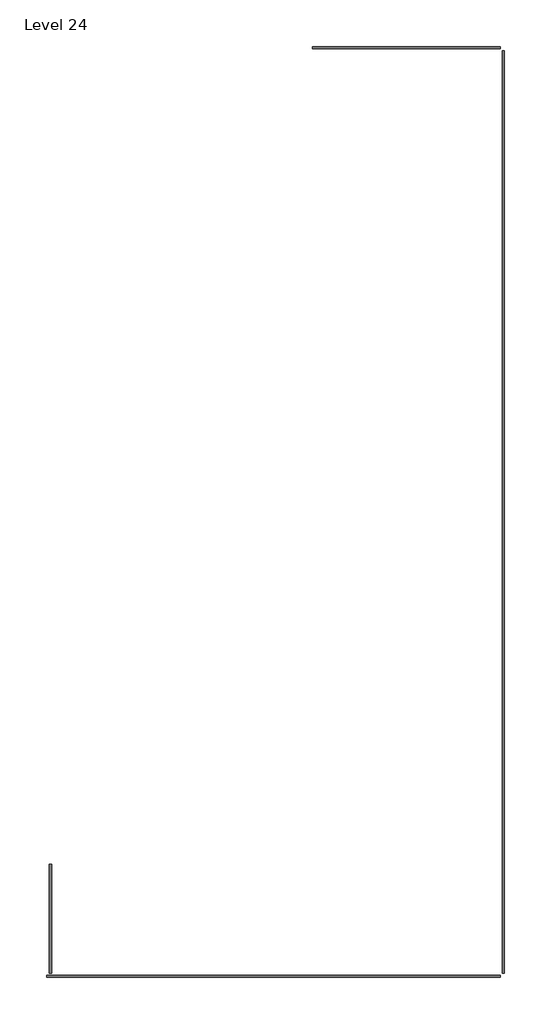
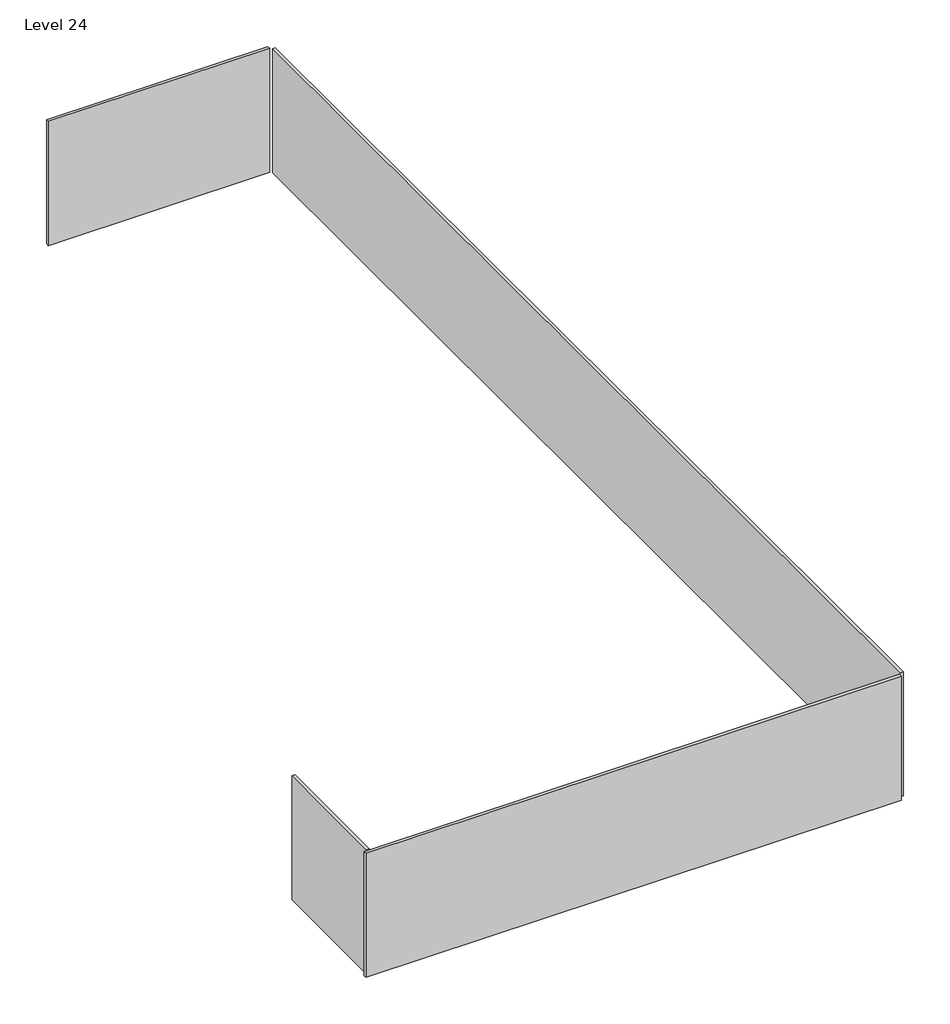
# One storey: 4 plates.
"""IFC4 building model written with IfcOpenShell, lengths in millimetres."""

from ifc_helpers import new_model, si_unit, origin, place, context, project, spatial, transform, mapped, element, save
from components import system_panel_glazed_5a380d23, system_panel_glazed_f6fb2dd6, system_panel_glazed_70773d7f, system_panel_glazed_2422818d

model = new_model("IFC4")

# Units and contexts
model_context = context("Model", 3, world=origin())
ifc_project = project(units=[si_unit("LENGTHUNIT", "METRE", prefix="MILLI")], contexts=[model_context])

# Site, building, storey
site = spatial("IfcSite", under=ifc_project)
building = spatial("IfcBuilding", under=site)
storey = spatial("IfcBuildingStorey", under=building, Name="Level 24", Elevation=39090.6)

# Plates
placement = place(None, origin())
system_panel_glazed_shape = system_panel_glazed_5a380d23(model_context)
element("IfcPlate", 1, ObjectType="System Panel : Glazed", at=placement, inside=storey, context=model_context, shape_type="MappedRepresentation", body=[
    mapped(system_panel_glazed_shape, transform((9019.0964352, -5911.0278294, 39090.6), x_axis=(1.0, 0.0, 0.0), y_axis=(0.0, 1.0, 0.0), z_axis=(0.0, 0.0, 1.0))),
])
system_panel_glazed_2_shape = system_panel_glazed_f6fb2dd6(model_context)
element("IfcPlate", 2, ObjectType="System Panel : Glazed", at=placement, inside=storey, context=model_context, shape_type="MappedRepresentation", body=[
    mapped(system_panel_glazed_2_shape, transform((5145.5964352, -15423.3278294, 39090.6), x_axis=(0.0, 1.0, 0.0), y_axis=(-1.0, 0.0, 0.0), z_axis=(0.0, 0.0, 1.0))),
])
system_panel_glazed_3_shape = system_panel_glazed_70773d7f(model_context)
element("IfcPlate", 3, ObjectType="System Panel : Glazed", at=placement, inside=storey, context=model_context, shape_type="MappedRepresentation", body=[
    mapped(system_panel_glazed_3_shape, transform((10047.7964352, -10965.6278294, 39090.6), x_axis=(0.0, -1.0, 0.0), y_axis=(1.0, 0.0, 0.0), z_axis=(0.0, 0.0, 1.0))),
])
system_panel_glazed_4_shape = system_panel_glazed_2422818d(model_context)
element("IfcPlate", 4, ObjectType="System Panel : Glazed", at=placement, inside=storey, context=model_context, shape_type="MappedRepresentation", body=[
    mapped(system_panel_glazed_4_shape, transform((7559.6180352, -16020.2278294, 39090.6), x_axis=(-1.0, 0.0, 0.0), y_axis=(0.0, -1.0, 0.0), z_axis=(0.0, 0.0, 1.0))),
])

save(model, "model.ifc")

# Revit data of these elements
# Type "System Panel : Glazed"
#   Construction Type Id = "GSP4R"
#   Analytic Construction = "1/8 in Pilkington single glazing"
#   Visual Light Transmittance = 0.9
#   Solar Heat Gain Coefficient = 0.86
#   Heat Transfer Coefficient (U) = 1.18115 BTU/(h·ft²·°F)
# Elements 1, 2, 3, 4 (IfcPlate, "System Panel : Glazed")
#   Phase Created = New Construction
#   Materials on its faces: "Glass"
# Materials
#   "Glass": class "Glass", colour RGB 0 128 192, transparency 0.75, Description = "Soda Lime Glass", Cost = 0
